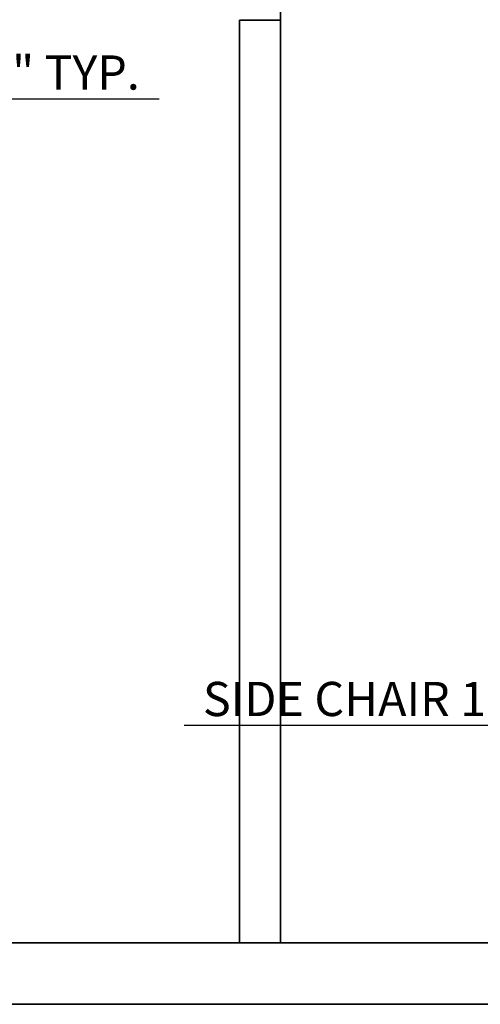
# Model space of a CAD drawing. Units: inches. Extents: x -100 to 766, y -562 to 63.
# Tile 6 of 11: x 380 to 448, y -467 to -323. Entities that reach past the tile are written whole.
import ezdxf

# ---------------------------------------------------------------- set-up
doc = ezdxf.new("R2010")
doc.units = ezdxf.units.IN
doc.layers.add('A-ANNO-DIMS', color=2, linetype='Continuous', lineweight=18)
doc.layers.add('A-WALL', color=7, linetype='Continuous', lineweight=35)
doc.styles.get("Standard").update_dxf_attribs({"font": 'arial.ttf'})
doc.dimstyles.new('ISO-25', dxfattribs={"dimtxt": 5, "dimasz": 5, "dimexe": 1.25, "dimexo": 0.625, "dimtad": 1, "dimlunit": 3, "dimtxsty": 'Standard', "dimcen": 2.5, "dimadec": 0, "dimazin": 0, "dimtfac": 1, "dimtmove": 0, "dimatfit": 3, "dimfxl": 1, "dimfxlon": 1, "dimarcsym": 0})

# ---------------------------------------------------------------- blocks, each defined once
blk = doc.blocks.new('*D24')
at = {"layer": 'A-ANNO-DIMS', "color": 0, "lineweight": -2, "transparency": 16777216}
for p, q in [((482.94, -425.44), (482.94, -427.69)), ((502.97, -425.44), (502.97, -427.69)), ((482.94, -426.44), (404.32, -426.44)), ((497.97, -426.44), (487.94, -426.44))]:
    blk.add_line(p, q, dxfattribs=at)
at = {"layer": 'A-ANNO-DIMS', "color": 0, "transparency": 16777216}
for points in [[(487.94, -425.61), (487.94, -427.28), (482.94, -426.44)], [(497.97, -425.61), (497.97, -427.28), (502.97, -426.44)]]:
    blk.add_solid(points, dxfattribs=at)
at = {"layer": 'Defpoints', "color": 0, "transparency": 16777216}
for p in [(482.94, -423.44), (502.97, -423.44), (482.94, -426.44)]:
    blk.add_point(p, dxfattribs=at)
at = {"layer": 'A-ANNO-DIMS', "color": 0, "transparency": 16777216, "insert": (441.13, -423.23), "char_height": 5, "attachment_point": 5, "rotation": 0}
blk.add_mtext('SIDE CHAIR 1\'-8" TYP.', dxfattribs=at)
blk = doc.blocks.new('*D32')
at = {"layer": 'A-ANNO-DIMS', "color": 0, "lineweight": -2, "transparency": 16777216}
for p, q in [((304.17, -335.87), (304.17, -333.62)), ((319.93, -335.87), (319.93, -333.62)), ((309.17, -334.87), (314.93, -334.87)), ((319.93, -334.87), (400.64, -334.87))]:
    blk.add_line(p, q, dxfattribs=at)
at = {"layer": 'A-ANNO-DIMS', "color": 0, "transparency": 16777216}
for points in [[(309.17, -334.04), (309.17, -335.71), (304.17, -334.87)], [(314.93, -334.04), (314.93, -335.71), (319.93, -334.87)]]:
    blk.add_solid(points, dxfattribs=at)
at = {"layer": 'Defpoints', "color": 0, "transparency": 16777216}
for p in [(319.93, -334.87), (304.17, -337.24), (319.93, -337.24)]:
    blk.add_point(p, dxfattribs=at)
at = {"layer": 'A-ANNO-DIMS', "color": 0, "transparency": 16777216, "insert": (362.79, -331.66), "char_height": 5, "attachment_point": 5}
blk.add_mtext('TASK CHAIR 1\'-4" TYP.', dxfattribs=at)
blk = doc.blocks.new('*D49')
at = {"layer": 'A-ANNO-DIMS', "color": 0, "lineweight": -2, "transparency": 16777216}
for p, q in [((-88.51, -356.21), (-90.76, -356.21)), ((-89.51, -361.21), (-89.51, -417.21)), ((-88.51, -422.21), (-90.76, -422.21))]:
    blk.add_line(p, q, dxfattribs=at)
at = {"layer": 'A-ANNO-DIMS', "color": 0, "transparency": 16777216}
for points in [[(-90.35, -361.21), (-88.68, -361.21), (-89.51, -356.21)], [(-90.35, -417.21), (-88.68, -417.21), (-89.51, -422.21)]]:
    blk.add_solid(points, dxfattribs=at)
at = {"layer": 'Defpoints', "color": 0, "transparency": 16777216}
for p in [(562.39, -356.21), (-89.51, -422.21), (562.39, -422.21)]:
    blk.add_point(p, dxfattribs=at)
at = {"layer": 'A-ANNO-DIMS', "color": 0, "transparency": 16777216, "insert": (-92.69, -389.21), "char_height": 5, "attachment_point": 5, "rotation": 90}
blk.add_mtext('5\'-6"', dxfattribs=at)
blk = doc.blocks.new('*D51')
at = {"layer": 'A-ANNO-DIMS', "color": 0, "lineweight": -2, "transparency": 16777216}
for p, q in [((-88.51, -308.21), (-90.76, -308.21)), ((-89.51, -313.21), (-89.51, -339.21)), ((-88.51, -344.21), (-90.76, -344.21))]:
    blk.add_line(p, q, dxfattribs=at)
at = {"layer": 'A-ANNO-DIMS', "color": 0, "transparency": 16777216}
for points in [[(-90.35, -313.21), (-88.68, -313.21), (-89.51, -308.21)], [(-90.35, -339.21), (-88.68, -339.21), (-89.51, -344.21)]]:
    blk.add_solid(points, dxfattribs=at)
at = {"layer": 'Defpoints', "color": 0, "transparency": 16777216}
for p in [(598.6, -308.21), (-89.51, -344.21), (598.6, -344.21)]:
    blk.add_point(p, dxfattribs=at)
at = {"layer": 'A-ANNO-DIMS', "color": 0, "transparency": 16777216, "insert": (-92.69, -326.21), "char_height": 5, "attachment_point": 5, "rotation": 90}
blk.add_mtext('3\'-0"', dxfattribs=at)
blk = doc.blocks.new('*D70')
at = {"layer": 'A-ANNO-DIMS', "color": 0, "lineweight": -2, "transparency": 16777216}
for p, q in [((-88.51, -376.85), (-90.76, -376.85)), ((-89.51, -381.85), (-89.51, -419.34)), ((-88.51, -424.34), (-90.76, -424.34))]:
    blk.add_line(p, q, dxfattribs=at)
at = {"layer": 'A-ANNO-DIMS', "color": 0, "transparency": 16777216}
for points in [[(-90.35, -381.85), (-88.68, -381.85), (-89.51, -376.85)], [(-90.35, -419.34), (-88.68, -419.34), (-89.51, -424.34)]]:
    blk.add_solid(points, dxfattribs=at)
at = {"layer": 'Defpoints', "color": 0, "transparency": 16777216}
for p in [(679.5, -376.85), (-89.51, -424.34), (679.5, -424.34)]:
    blk.add_point(p, dxfattribs=at)
at = {"layer": 'A-ANNO-DIMS', "color": 0, "transparency": 16777216, "insert": (-92.73, -400.59), "char_height": 5, "attachment_point": 5, "rotation": 90}
blk.add_mtext('3\'-11 1/2"', dxfattribs=at)
blk = doc.blocks.new('*D73')
at = {"layer": 'A-ANNO-DIMS', "color": 0, "lineweight": -2, "transparency": 16777216}
for p, q in [((-88.51, -345.04), (-90.76, -345.04)), ((-89.51, -350.04), (-89.51, -401.82)), ((-88.51, -406.82), (-90.76, -406.82))]:
    blk.add_line(p, q, dxfattribs=at)
at = {"layer": 'A-ANNO-DIMS', "color": 0, "transparency": 16777216}
for points in [[(-90.35, -350.04), (-88.68, -350.04), (-89.51, -345.04)], [(-90.35, -401.82), (-88.68, -401.82), (-89.51, -406.82)]]:
    blk.add_solid(points, dxfattribs=at)
at = {"layer": 'Defpoints', "color": 0, "transparency": 16777216}
for p in [(475.3, -345.04), (-89.51, -406.82), (475.3, -406.82)]:
    blk.add_point(p, dxfattribs=at)
at = {"layer": 'A-ANNO-DIMS', "color": 0, "transparency": 16777216, "insert": (-92.69, -375.93), "char_height": 5, "attachment_point": 5, "rotation": 90}
blk.add_mtext('5\'-2"', dxfattribs=at)
blk = doc.blocks.new('*D83')
at = {"layer": 'A-ANNO-DIMS', "color": 0, "lineweight": -2, "transparency": 16777216}
for p, q in [((-88.51, -422.21), (-90.76, -422.21)), ((-89.51, -427.21), (-89.51, -453.21)), ((-88.51, -458.21), (-90.76, -458.21))]:
    blk.add_line(p, q, dxfattribs=at)
at = {"layer": 'A-ANNO-DIMS', "color": 0, "transparency": 16777216}
for points in [[(-90.35, -427.21), (-88.68, -427.21), (-89.51, -422.21)], [(-90.35, -453.21), (-88.68, -453.21), (-89.51, -458.21)]]:
    blk.add_solid(points, dxfattribs=at)
at = {"layer": 'Defpoints', "color": 0, "transparency": 16777216}
for p in [(562.39, -422.21), (-89.51, -458.21), (562.39, -458.21)]:
    blk.add_point(p, dxfattribs=at)
at = {"layer": 'A-ANNO-DIMS', "color": 0, "transparency": 16777216, "insert": (-92.69, -440.21), "char_height": 5, "attachment_point": 5, "rotation": 90}
blk.add_mtext('3\'-0"', dxfattribs=at)

msp = doc.modelspace()

# ---------------------------------------------------------------- linework, layer by layer
at = {"layer": 'A-WALL'}
for p, q in [((418.394, -458.214), (418.394, -272.214)), ((412.394, -458.214), (412.394, -323.377)), ((412.394, -323.377), (418.394, -323.377)), ((532.388, -458.214), (250.388, -458.214))]:
    msp.add_line(p, q, dxfattribs=at)
msp.add_lwpolyline([(1.388, 12.786), (721.388, 12.786), (721.388, -467.214), (1.388, -467.214)], close=True, dxfattribs=at)

# ---------------------------------------------------------------- dimensions: what is measured, and where the dimension line sits
at = {"layer": 'A-ANNO-DIMS'}
for base, p1, p2, picture, middle in [((-89.513, -344.214), (598.603, -308.214), (598.603, -344.214), '*D51', (-92.693, -326.214)), ((-89.513, -406.822), (475.3, -345.045), (475.3, -406.822), '*D73', (-92.691, -375.933)), ((-89.513, -422.214), (562.394, -356.214), (562.394, -422.214), '*D49', (-92.691, -389.214)), ((-89.513, -424.336), (679.495, -376.848), (679.495, -424.336), '*D70', (-92.725, -400.592)), ((-89.513, -458.214), (562.394, -422.214), (562.394, -458.214), '*D83', (-92.693, -440.214))]:
    dim = msp.add_linear_dim(base=base, p1=p1, p2=p2, angle=90, dimstyle='ISO-25', override={"dimdec": 1, "dimlfac": 1, "dimrnd": 0, "dimzin": 1, "dimdsep": 46, "dimlunit": 4, "dimfrac": 2}, dxfattribs=at)
    dim.commit()
    dim.dimension.update_dxf_attribs({"geometry": picture, "text_midpoint": middle})
dim = msp.add_linear_dim(base=(319.931, -334.874), p1=(304.173, -337.238), p2=(319.931, -337.238), text='TASK CHAIR <> TYP.', dimstyle='ISO-25', override={"dimdec": 1, "dimlfac": 1, "dimrnd": 0, "dimzin": 1, "dimdsep": 46, "dimlunit": 4, "dimfrac": 2}, dxfattribs=at)
dim.commit()
dim.dimension.update_dxf_attribs({"geometry": '*D32', "text_midpoint": (362.787, -331.664)})
dim = msp.add_linear_dim(base=(482.936, -426.444), p1=(502.965, -423.44), p2=(482.936, -423.44), angle=180, text='SIDE CHAIR <> TYP.', dimstyle='ISO-25', override={"dimdec": 1, "dimlfac": 1, "dimrnd": 0, "dimzin": 1, "dimdsep": 46, "dimlunit": 4, "dimfrac": 2}, dxfattribs=at)
dim.commit()
dim.dimension.update_dxf_attribs({"geometry": '*D24', "text_midpoint": (441.126, -423.234)})

doc.saveas('drawing.dxf')
